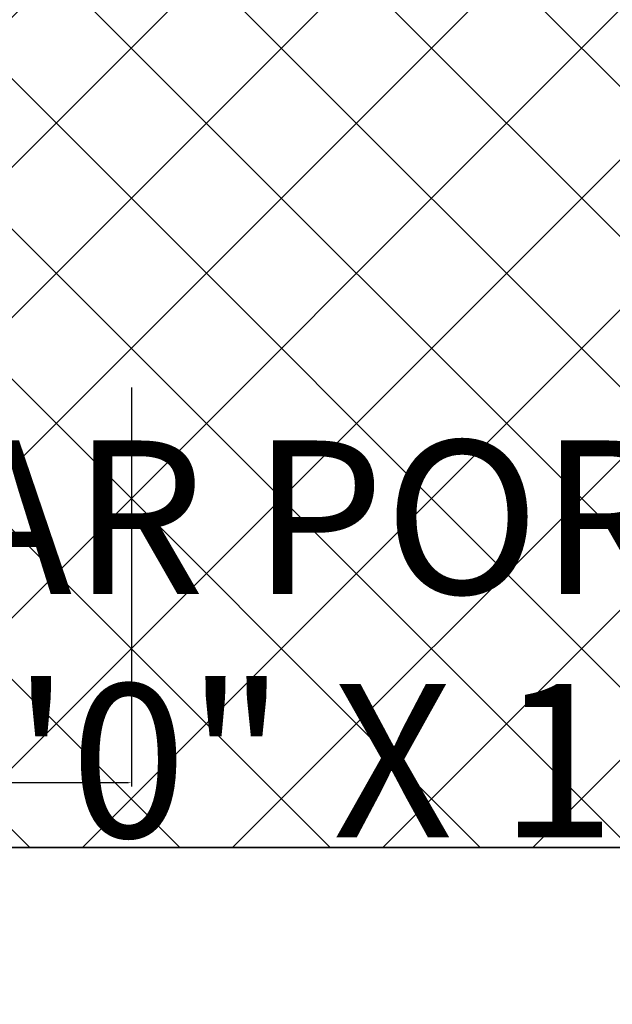
# Model space of a CAD drawing. Units: inches. Extents: x 2167 to 2589, y 1680 to 2489.
# Tile 6 of 38: x 2307 to 2335, y 1680 to 1727. Entities that reach past the tile are written whole.
import ezdxf

# ---------------------------------------------------------------- set-up
doc = ezdxf.new("R2010")
doc.units = ezdxf.units.IN
doc.header["$MEASUREMENT"] = 0
for name, color, linetype, lineweight in [('A-ANNO-DIMS', 2, 'Continuous', 18), ('A-AREA-IDEN', 7, 'Continuous', 18), ('C-PROP', 7, 'Continuous', 35), ('L-PVMT-PATT', 252, 'Continuous', 13)]:
    doc.layers.add(name, color=color, linetype=linetype, lineweight=lineweight)
doc.styles.get("Standard").update_dxf_attribs({"font": 'arial.ttf'})
doc.dimstyles.get("Standard").update_dxf_attribs({"dimtxt": 7, "dimasz": 0.18, "dimexe": 0.18, "dimexo": 0.0625, "dimgap": 0.09, "dimtad": 0, "dimtih": 1, "dimtoh": 1, "dimdec": 1, "dimzin": 0, "dimdsep": 46, "dimlunit": 3, "dimtxsty": 'Standard', "dimcen": 0.09, "dimadec": 0, "dimazin": 0, "dimtfac": 1, "dimtdec": 1, "dimtofl": 0, "dimtmove": 0, "dimatfit": 3, "dimfxl": 1, "dimtolj": 1, "dimtzin": 0, "dimarcsym": 0})

# ---------------------------------------------------------------- blocks, each defined once
blk = doc.blocks.new('*D46')
at = {"layer": 'A-ANNO-DIMS', "color": 0, "lineweight": -2, "transparency": 16777216}
for p, q in [((2251.218, 1709.362), (2251.218, 1690.565)), ((2312.254, 1709.362), (2312.254, 1690.565)), ((2251.398, 1690.745), (2260.312, 1690.745)), ((2312.074, 1690.745), (2303.16, 1690.745))]:
    blk.add_line(p, q, dxfattribs=at)
at = {"layer": 'A-ANNO-DIMS', "color": 0, "transparency": 16777216}
for points in [[(2251.398, 1690.775), (2251.398, 1690.715), (2251.218, 1690.745)], [(2312.074, 1690.775), (2312.074, 1690.715), (2312.254, 1690.745)]]:
    blk.add_solid(points, dxfattribs=at)
at = {"layer": 'Defpoints', "color": 0, "transparency": 16777216}
for p in [(2251.218, 1709.425), (2312.254, 1709.425), (2312.254, 1690.745)]:
    blk.add_point(p, dxfattribs=at)
at = {"layer": 'A-ANNO-DIMS', "color": 0, "transparency": 16777216, "insert": (2281.736, 1690.745), "char_height": 7, "attachment_point": 5}
blk.add_mtext('\\A1;5\'-1" TYP.', dxfattribs=at)

msp = doc.modelspace()

# ---------------------------------------------------------------- hatches: boundary and pattern name
at = {"layer": 'L-PVMT-PATT'}
h = msp.add_hatch(dxfattribs=at)
h.set_pattern_fill('ANSI37', color=256, scale=40)
h.paths.add_polyline_path([(2417.548, 1783.695), (2417.548, 1846.042), (2239.361, 1846.042), (2239.361, 1687.695), (2369.843, 1687.695), (2369.843, 1696.695), (2375.607, 1696.695), (2416.107, 1696.695), (2417.548, 1696.695)])

# ---------------------------------------------------------------- linework, layer by layer
at = {"layer": 'C-PROP'}
msp.add_line((2575.048, 1687.695), (2215.048, 1687.695), dxfattribs=at)

# ---------------------------------------------------------------- texts
at = {"layer": 'A-AREA-IDEN'}
for s, height, p in [('CAR PORCH', 7.2272, (2297.172, 1699.634)), ('16\'0" X 16\'0"', 7.22716, (2295.694, 1688.165))]:
    msp.add_text(s, height=height, dxfattribs=at).set_placement(p)

# ---------------------------------------------------------------- dimensions: what is measured, and where the dimension line sits
at = {"layer": 'A-ANNO-DIMS'}
dim = msp.add_linear_dim(base=(2312.254, 1690.745), p1=(2251.218, 1709.425), p2=(2312.254, 1709.425), text='<> TYP.', dimstyle='Standard', override={"dimdec": 1, "dimlfac": 1, "dimrnd": 0, "dimzin": 1, "dimdsep": 46, "dimlunit": 4, "dimfrac": 2}, dxfattribs=at)
dim.commit()
dim.dimension.update_dxf_attribs({"geometry": '*D46', "text_midpoint": (2281.736, 1690.745)})

doc.saveas('drawing.dxf')
